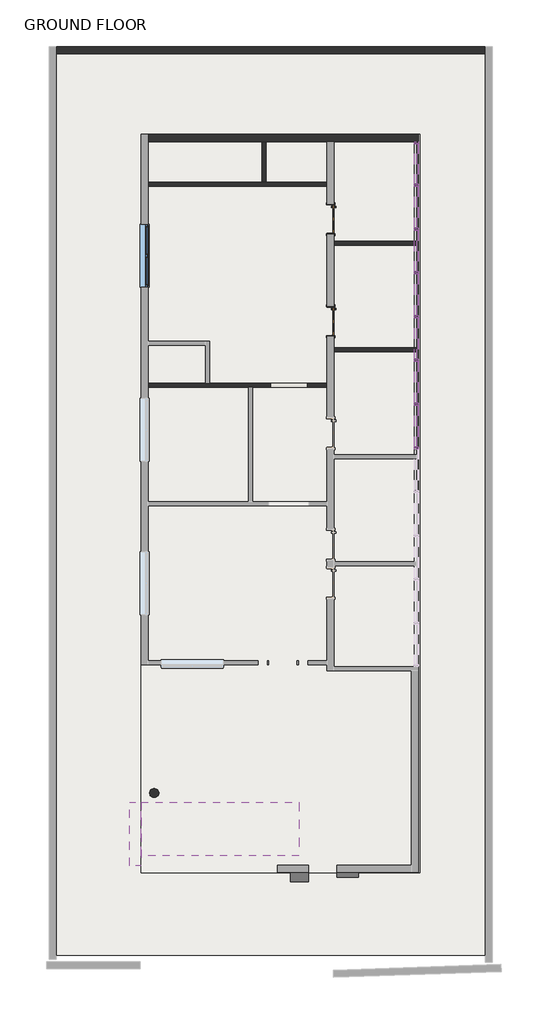
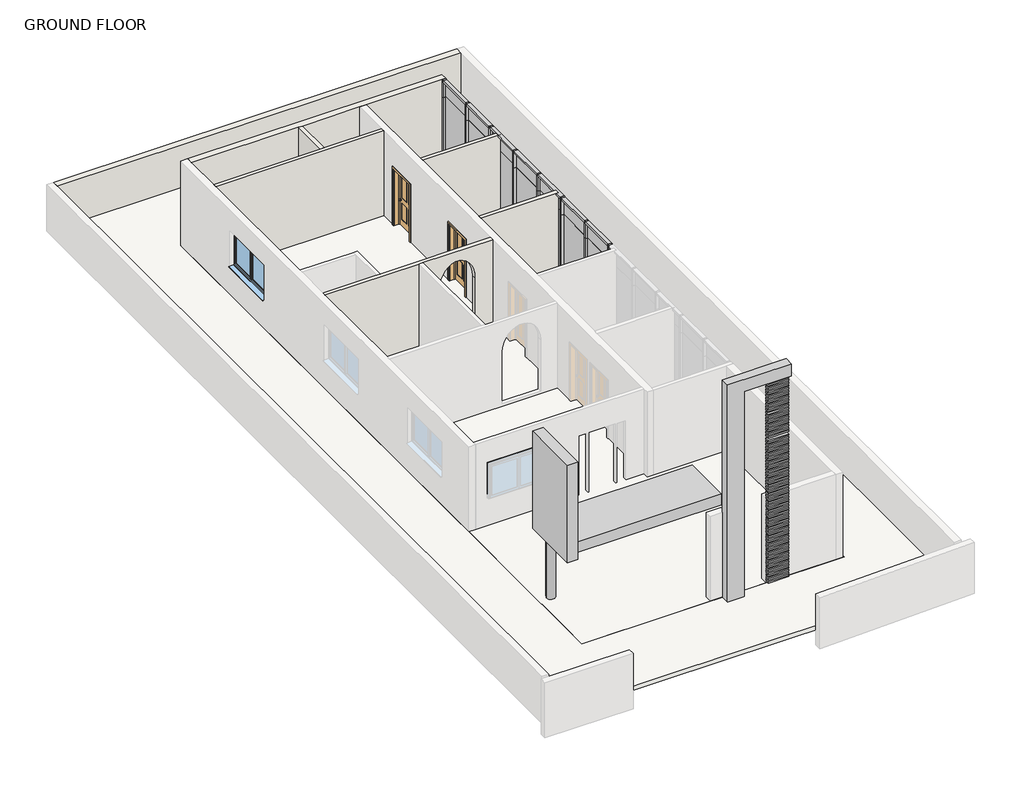
# One storey, part 2 of 2: 31 members, 14 plates, 7 walls, 4 proxies, 2 doors, 2 slabs, 1 column, 1 window.
"""IFC4 building model written with IfcOpenShell, lengths in millimetres."""

from ifc_helpers import new_model, si_unit, point, frame, origin, origin_with_axes, place, context, project, spatial, polyline, ellipse_curve, trimmed, outline, extrude, faceted_brep, transform, mapped, element, save
from ifc_brep_helpers import plane_surface, extruded_surface, advanced_brep
from components import generic_models_11_generic_models_11_3010cca1, generic_models_13_generic_models_13_f044a1e7, generic_models_2_generic_models_2_70f3bfce, generic_models_3_generic_models_3_1afd715e, round_column_column_1_x_1_3d9dadd9, door_8a5afc22, member_fe35c162, member_c919ac1a, member_f0fea5a5, member_6e77e263, member_47bfaf8a, member_ee409385, system_panel_glazed_23a28a9f, system_panel_glazed_17e06366, system_panel_glazed_701ad94b, system_panel_glazed_1ceb456a, w2_0001_w2_7b90d420

model = new_model("IFC4")

# Units and contexts
model_context = context("Model", 3, world=origin())
ifc_project = project(units=[si_unit("LENGTHUNIT", "METRE", prefix="MILLI")], contexts=[model_context])

# Site, building, storey
site = spatial("IfcSite", under=ifc_project)
building = spatial("IfcBuilding", under=site)
storey = spatial("IfcBuildingStorey", under=building, Name="GROUND FLOOR", Elevation=304.8)

# Proxies
placement = place(None, origin())
generic_models_11_generic_models_11_shape = generic_models_11_generic_models_11_3010cca1(model_context)
element("IfcBuildingElementProxy", 1, Name="Generic Models 11 : Generic Models 11", ObjectType="Generic Models 11 : Generic Models 11", at=placement, inside=storey, context=model_context, shape_type="MappedRepresentation", body=[
    mapped(generic_models_11_generic_models_11_shape, transform((0.0, 0.0, 0.0), x_axis=(1.0, 0.0, 0.0), y_axis=(0.0, 1.0, 0.0), z_axis=(0.0, 0.0, 1.0))),
])
generic_models_13_generic_models_13_shape = generic_models_13_generic_models_13_f044a1e7(model_context)
element("IfcBuildingElementProxy", 2, Name="Generic Models 13 : Generic Models 13", ObjectType="Generic Models 13 : Generic Models 13", at=placement, inside=storey, context=model_context, shape_type="MappedRepresentation", body=[
    mapped(generic_models_13_generic_models_13_shape, transform((0.0, 0.0, 0.0), x_axis=(1.0, 0.0, 0.0), y_axis=(0.0, 1.0, 0.0), z_axis=(0.0, 0.0, 1.0))),
])
generic_models_2_generic_models_2_shape = generic_models_2_generic_models_2_70f3bfce(model_context)
element("IfcBuildingElementProxy", 3, Name="Generic Models 2 : Generic Models 2", ObjectType="Generic Models 2 : Generic Models 2", at=placement, inside=storey, context=model_context, shape_type="MappedRepresentation", body=[
    mapped(generic_models_2_generic_models_2_shape, transform((0.0, 0.0, 0.0), x_axis=(1.0, 0.0, 0.0), y_axis=(0.0, 1.0, 0.0), z_axis=(0.0, 0.0, 1.0))),
])
generic_models_3_generic_models_3_shape = generic_models_3_generic_models_3_1afd715e(model_context)
element("IfcBuildingElementProxy", 4, Name="Generic Models 3 : Generic Models 3", ObjectType="Generic Models 3 : Generic Models 3", at=placement, inside=storey, context=model_context, shape_type="MappedRepresentation", body=[
    mapped(generic_models_3_generic_models_3_shape, transform((0.0, 0.0, 0.0), x_axis=(1.0, 0.0, 0.0), y_axis=(0.0, 1.0, 0.0), z_axis=(0.0, 0.0, 1.0))),
])

# Column
round_column_column_1_x_1_shape = round_column_column_1_x_1_3d9dadd9(model_context)
element("IfcColumn", 5, ObjectType="Round Column : COLUMN 1' X 1'", at=placement, inside=storey, context=model_context, shape_type="MappedRepresentation", body=[
    mapped(round_column_column_1_x_1_shape, transform((1692.4423568, -10961.9073314, 0.0), x_axis=(1.0, 0.0, 0.0), y_axis=(0.0, 1.0, 0.0), z_axis=(0.0, 0.0, 1.0))),
])

# Doors
door_shape = door_8a5afc22(model_context)
element("IfcDoor", 6, ObjectType="Door-Interior-Single-4_Panel-Wood : 36\" x 80\"", at=placement, inside=storey, context=model_context, shape_type="MappedRepresentation", body=[
    mapped(door_shape, transform((7334.4173568, 4100.2926686, 304.8), x_axis=(0.0, -1.0, 0.0), y_axis=(1.0, 0.0, 0.0), z_axis=(0.0, 0.0, 1.0))),
])
element("IfcDoor", 7, ObjectType="Door-Interior-Single-4_Panel-Wood : 36\" x 80\"", at=placement, inside=storey, context=model_context, shape_type="MappedRepresentation", body=[
    mapped(door_shape, transform((7334.4173568, 7364.1926686, 304.8), x_axis=(0.0, -1.0, 0.0), y_axis=(1.0, 0.0, 0.0), z_axis=(0.0, 0.0, 1.0))),
])

# Members
member_shape = member_fe35c162(model_context)
element("IfcMember", 8, ObjectType="Rectangular Mullion : 2.5\" x 5\" rectangular", at=placement, inside=storey, context=model_context, shape_type="MappedRepresentation", body=[
    mapped(member_shape, transform((10074.4423568, 9777.1926686, 304.8), x_axis=(0.0, 0.0, -1.0), y_axis=(-1.0, 0.0, 0.0), z_axis=(0.0, 1.0, 0.0))),
])
element("IfcMember", 9, ObjectType="Rectangular Mullion : 2.5\" x 5\" rectangular", at=placement, inside=storey, context=model_context, shape_type="MappedRepresentation", body=[
    mapped(member_shape, transform((10074.4423568, 8474.384335, 3352.8), x_axis=(0.0, 0.0, 1.0), y_axis=(-1.0, 0.0, 0.0), z_axis=(0.0, -1.0, 0.0))),
])
member_2_shape = member_c919ac1a(model_context)
element("IfcMember", 10, ObjectType="Rectangular Mullion : 2.5\" x 5\" rectangular", at=placement, inside=storey, context=model_context, shape_type="MappedRepresentation", body=[
    mapped(member_2_shape, transform((10074.4423568, 7076.3260017, 3352.8), x_axis=(0.0, 0.0, 1.0), y_axis=(-1.0, 0.0, 0.0), z_axis=(0.0, -1.0, 0.0))),
])
element("IfcMember", 11, ObjectType="Rectangular Mullion : 2.5\" x 5\" rectangular", at=placement, inside=storey, context=model_context, shape_type="MappedRepresentation", body=[
    mapped(member_2_shape, transform((10074.4423568, 5678.2676685, 3352.8), x_axis=(0.0, 0.0, 1.0), y_axis=(-1.0, 0.0, 0.0), z_axis=(0.0, -1.0, 0.0))),
])
element("IfcMember", 12, ObjectType="Rectangular Mullion : 2.5\" x 5\" rectangular", at=placement, inside=storey, context=model_context, shape_type="MappedRepresentation", body=[
    mapped(member_2_shape, transform((10074.4423568, 4280.2093352, 3352.8), x_axis=(0.0, 0.0, 1.0), y_axis=(-1.0, 0.0, 0.0), z_axis=(0.0, -1.0, 0.0))),
])
element("IfcMember", 13, ObjectType="Rectangular Mullion : 2.5\" x 5\" rectangular", at=placement, inside=storey, context=model_context, shape_type="MappedRepresentation", body=[
    mapped(member_2_shape, transform((10074.4423568, 2882.1510019, 3352.8), x_axis=(0.0, 0.0, 1.0), y_axis=(-1.0, 0.0, 0.0), z_axis=(0.0, -1.0, 0.0))),
])
element("IfcMember", 14, ObjectType="Rectangular Mullion : 2.5\" x 5\" rectangular", at=placement, inside=storey, context=model_context, shape_type="MappedRepresentation", body=[
    mapped(member_2_shape, transform((10074.4423568, 1484.0926686, 3352.8), x_axis=(0.0, 0.0, 1.0), y_axis=(-1.0, 0.0, 0.0), z_axis=(0.0, -1.0, 0.0))),
])
element("IfcMember", 15, ObjectType="Rectangular Mullion : 2.5\" x 5\" rectangular", at=placement, inside=storey, context=model_context, shape_type="MappedRepresentation", body=[
    mapped(member_2_shape, transform((10074.4423568, 86.0343353, 3352.8), x_axis=(0.0, 0.0, 1.0), y_axis=(-1.0, 0.0, 0.0), z_axis=(0.0, -1.0, 0.0))),
])
element("IfcMember", 16, ObjectType="Rectangular Mullion : 2.5\" x 5\" rectangular", at=placement, inside=storey, context=model_context, shape_type="MappedRepresentation", body=[
    mapped(member_2_shape, transform((10074.4423568, 8410.884335, 304.8), x_axis=(0.0, 0.0, -1.0), y_axis=(-1.0, 0.0, 0.0), z_axis=(0.0, 1.0, 0.0))),
])
element("IfcMember", 17, ObjectType="Rectangular Mullion : 2.5\" x 5\" rectangular", at=placement, inside=storey, context=model_context, shape_type="MappedRepresentation", body=[
    mapped(member_2_shape, transform((10074.4423568, 7012.8260017, 304.8), x_axis=(0.0, 0.0, -1.0), y_axis=(-1.0, 0.0, 0.0), z_axis=(0.0, 1.0, 0.0))),
])
element("IfcMember", 18, ObjectType="Rectangular Mullion : 2.5\" x 5\" rectangular", at=placement, inside=storey, context=model_context, shape_type="MappedRepresentation", body=[
    mapped(member_2_shape, transform((10074.4423568, 5614.7676685, 304.8), x_axis=(0.0, 0.0, -1.0), y_axis=(-1.0, 0.0, 0.0), z_axis=(0.0, 1.0, 0.0))),
])
element("IfcMember", 19, ObjectType="Rectangular Mullion : 2.5\" x 5\" rectangular", at=placement, inside=storey, context=model_context, shape_type="MappedRepresentation", body=[
    mapped(member_2_shape, transform((10074.4423568, 4216.7093352, 304.8), x_axis=(0.0, 0.0, -1.0), y_axis=(-1.0, 0.0, 0.0), z_axis=(0.0, 1.0, 0.0))),
])
element("IfcMember", 20, ObjectType="Rectangular Mullion : 2.5\" x 5\" rectangular", at=placement, inside=storey, context=model_context, shape_type="MappedRepresentation", body=[
    mapped(member_2_shape, transform((10074.4423568, 2818.6510019, 304.8), x_axis=(0.0, 0.0, -1.0), y_axis=(-1.0, 0.0, 0.0), z_axis=(0.0, 1.0, 0.0))),
])
element("IfcMember", 21, ObjectType="Rectangular Mullion : 2.5\" x 5\" rectangular", at=placement, inside=storey, context=model_context, shape_type="MappedRepresentation", body=[
    mapped(member_2_shape, transform((10074.4423568, 1420.5926686, 304.8), x_axis=(0.0, 0.0, -1.0), y_axis=(-1.0, 0.0, 0.0), z_axis=(0.0, 1.0, 0.0))),
])
element("IfcMember", 22, ObjectType="Rectangular Mullion : 2.5\" x 5\" rectangular", at=placement, inside=storey, context=model_context, shape_type="MappedRepresentation", body=[
    mapped(member_2_shape, transform((10074.4423568, 22.5343353, 304.8), x_axis=(0.0, 0.0, -1.0), y_axis=(-1.0, 0.0, 0.0), z_axis=(0.0, 1.0, 0.0))),
])
member_3_shape = member_f0fea5a5(model_context)
element("IfcMember", 23, ObjectType="Rectangular Mullion : 2.5\" x 5\" rectangular", at=placement, inside=storey, context=model_context, shape_type="MappedRepresentation", body=[
    mapped(member_3_shape, transform((10074.4423568, 8442.634335, 304.8), x_axis=(0.0, -1.0, 0.0), y_axis=(-1.0, 0.0, 0.0), z_axis=(0.0, 0.0, -1.0))),
])
element("IfcMember", 24, ObjectType="Rectangular Mullion : 2.5\" x 5\" rectangular", at=placement, inside=storey, context=model_context, shape_type="MappedRepresentation", body=[
    mapped(member_3_shape, transform((10074.4423568, 7044.5760017, 304.8), x_axis=(0.0, -1.0, 0.0), y_axis=(-1.0, 0.0, 0.0), z_axis=(0.0, 0.0, -1.0))),
])
element("IfcMember", 25, ObjectType="Rectangular Mullion : 2.5\" x 5\" rectangular", at=placement, inside=storey, context=model_context, shape_type="MappedRepresentation", body=[
    mapped(member_3_shape, transform((10074.4423568, 5646.5176685, 304.8), x_axis=(0.0, -1.0, 0.0), y_axis=(-1.0, 0.0, 0.0), z_axis=(0.0, 0.0, -1.0))),
])
element("IfcMember", 26, ObjectType="Rectangular Mullion : 2.5\" x 5\" rectangular", at=placement, inside=storey, context=model_context, shape_type="MappedRepresentation", body=[
    mapped(member_3_shape, transform((10074.4423568, 4248.4593352, 304.8), x_axis=(0.0, -1.0, 0.0), y_axis=(-1.0, 0.0, 0.0), z_axis=(0.0, 0.0, -1.0))),
])
element("IfcMember", 27, ObjectType="Rectangular Mullion : 2.5\" x 5\" rectangular", at=placement, inside=storey, context=model_context, shape_type="MappedRepresentation", body=[
    mapped(member_3_shape, transform((10074.4423568, 2850.4010019, 304.8), x_axis=(0.0, -1.0, 0.0), y_axis=(-1.0, 0.0, 0.0), z_axis=(0.0, 0.0, -1.0))),
])
element("IfcMember", 28, ObjectType="Rectangular Mullion : 2.5\" x 5\" rectangular", at=placement, inside=storey, context=model_context, shape_type="MappedRepresentation", body=[
    mapped(member_3_shape, transform((10074.4423568, 1452.3426686, 304.8), x_axis=(0.0, -1.0, 0.0), y_axis=(-1.0, 0.0, 0.0), z_axis=(0.0, 0.0, -1.0))),
])
element("IfcMember", 29, ObjectType="Rectangular Mullion : 2.5\" x 5\" rectangular", at=placement, inside=storey, context=model_context, shape_type="MappedRepresentation", body=[
    mapped(member_3_shape, transform((10074.4423568, 54.2843353, 304.8), x_axis=(0.0, -1.0, 0.0), y_axis=(-1.0, 0.0, 0.0), z_axis=(0.0, 0.0, -1.0))),
])
member_4_shape = member_6e77e263(model_context)
element("IfcMember", 30, ObjectType="Rectangular Mullion : 2.5\" x 5\" rectangular", at=placement, inside=storey, context=model_context, shape_type="MappedRepresentation", body=[
    mapped(member_4_shape, transform((10074.4423568, 8442.634335, 2743.2), x_axis=(0.0, -1.0, 0.0), y_axis=(-1.0, 0.0, 0.0), z_axis=(0.0, 0.0, -1.0))),
])
element("IfcMember", 31, ObjectType="Rectangular Mullion : 2.5\" x 5\" rectangular", at=placement, inside=storey, context=model_context, shape_type="MappedRepresentation", body=[
    mapped(member_4_shape, transform((10074.4423568, 7044.5760017, 2743.2), x_axis=(0.0, -1.0, 0.0), y_axis=(-1.0, 0.0, 0.0), z_axis=(0.0, 0.0, -1.0))),
])
element("IfcMember", 32, ObjectType="Rectangular Mullion : 2.5\" x 5\" rectangular", at=placement, inside=storey, context=model_context, shape_type="MappedRepresentation", body=[
    mapped(member_4_shape, transform((10074.4423568, 5646.5176685, 2743.2), x_axis=(0.0, -1.0, 0.0), y_axis=(-1.0, 0.0, 0.0), z_axis=(0.0, 0.0, -1.0))),
])
element("IfcMember", 33, ObjectType="Rectangular Mullion : 2.5\" x 5\" rectangular", at=placement, inside=storey, context=model_context, shape_type="MappedRepresentation", body=[
    mapped(member_4_shape, transform((10074.4423568, 4248.4593352, 2743.2), x_axis=(0.0, -1.0, 0.0), y_axis=(-1.0, 0.0, 0.0), z_axis=(0.0, 0.0, -1.0))),
])
element("IfcMember", 34, ObjectType="Rectangular Mullion : 2.5\" x 5\" rectangular", at=placement, inside=storey, context=model_context, shape_type="MappedRepresentation", body=[
    mapped(member_4_shape, transform((10074.4423568, 2850.4010019, 2743.2), x_axis=(0.0, -1.0, 0.0), y_axis=(-1.0, 0.0, 0.0), z_axis=(0.0, 0.0, -1.0))),
])
element("IfcMember", 35, ObjectType="Rectangular Mullion : 2.5\" x 5\" rectangular", at=placement, inside=storey, context=model_context, shape_type="MappedRepresentation", body=[
    mapped(member_4_shape, transform((10074.4423568, 1452.3426686, 2743.2), x_axis=(0.0, -1.0, 0.0), y_axis=(-1.0, 0.0, 0.0), z_axis=(0.0, 0.0, -1.0))),
])
element("IfcMember", 36, ObjectType="Rectangular Mullion : 2.5\" x 5\" rectangular", at=placement, inside=storey, context=model_context, shape_type="MappedRepresentation", body=[
    mapped(member_4_shape, transform((10074.4423568, 54.2843353, 2743.2), x_axis=(0.0, -1.0, 0.0), y_axis=(-1.0, 0.0, 0.0), z_axis=(0.0, 0.0, -1.0))),
])
member_5_shape = member_47bfaf8a(model_context)
element("IfcMember", 37, ObjectType="Rectangular Mullion : 2.5\" x 5\" rectangular", at=placement, inside=storey, context=model_context, shape_type="MappedRepresentation", body=[
    mapped(member_5_shape, transform((10074.4423568, 9840.6926686, 3352.8), x_axis=(0.0, 1.0, 0.0), y_axis=(-1.0, 0.0, 0.0), z_axis=(0.0, 0.0, 1.0))),
])
member_6_shape = member_ee409385(model_context)
element("IfcMember", 38, ObjectType="Rectangular Mullion : 2.5\" x 5\" rectangular", at=placement, inside=storey, context=model_context, shape_type="MappedRepresentation", body=[
    mapped(member_6_shape, transform((10074.4423568, 9840.6926686, 2743.2), x_axis=(0.0, 1.0, 0.0), y_axis=(-1.0, 0.0, 0.0), z_axis=(0.0, 0.0, 1.0))),
])

# Plates
system_panel_glazed_shape = system_panel_glazed_23a28a9f(model_context)
element("IfcPlate", 39, ObjectType="System Panel : Glazed", at=placement, inside=storey, context=model_context, shape_type="MappedRepresentation", body=[
    mapped(system_panel_glazed_shape, transform((10074.4423568, 9125.7885018, 368.3), x_axis=(0.0, -1.0, 0.0), y_axis=(1.0, 0.0, 0.0), z_axis=(0.0, 0.0, 1.0))),
])
system_panel_glazed_2_shape = system_panel_glazed_17e06366(model_context)
element("IfcPlate", 40, ObjectType="System Panel : Glazed", at=placement, inside=storey, context=model_context, shape_type="MappedRepresentation", body=[
    mapped(system_panel_glazed_2_shape, transform((10074.4423568, 9125.7885018, 2743.2), x_axis=(0.0, -1.0, 0.0), y_axis=(1.0, 0.0, 0.0), z_axis=(0.0, 0.0, 1.0))),
])
system_panel_glazed_3_shape = system_panel_glazed_701ad94b(model_context)
element("IfcPlate", 41, ObjectType="System Panel : Glazed", at=placement, inside=storey, context=model_context, shape_type="MappedRepresentation", body=[
    mapped(system_panel_glazed_3_shape, transform((10074.4423568, 7743.6051684, 368.3), x_axis=(0.0, -1.0, 0.0), y_axis=(1.0, 0.0, 0.0), z_axis=(0.0, 0.0, 1.0))),
])
element("IfcPlate", 42, ObjectType="System Panel : Glazed", at=placement, inside=storey, context=model_context, shape_type="MappedRepresentation", body=[
    mapped(system_panel_glazed_3_shape, transform((10074.4423568, 6345.5468351, 368.3), x_axis=(0.0, -1.0, 0.0), y_axis=(1.0, 0.0, 0.0), z_axis=(0.0, 0.0, 1.0))),
])
element("IfcPlate", 43, ObjectType="System Panel : Glazed", at=placement, inside=storey, context=model_context, shape_type="MappedRepresentation", body=[
    mapped(system_panel_glazed_3_shape, transform((10074.4423568, 4947.4885018, 368.3), x_axis=(0.0, -1.0, 0.0), y_axis=(1.0, 0.0, 0.0), z_axis=(0.0, 0.0, 1.0))),
])
element("IfcPlate", 44, ObjectType="System Panel : Glazed", at=placement, inside=storey, context=model_context, shape_type="MappedRepresentation", body=[
    mapped(system_panel_glazed_3_shape, transform((10074.4423568, 3549.4301685, 368.3), x_axis=(0.0, -1.0, 0.0), y_axis=(1.0, 0.0, 0.0), z_axis=(0.0, 0.0, 1.0))),
])
element("IfcPlate", 45, ObjectType="System Panel : Glazed", at=placement, inside=storey, context=model_context, shape_type="MappedRepresentation", body=[
    mapped(system_panel_glazed_3_shape, transform((10074.4423568, 2151.3718352, 368.3), x_axis=(0.0, -1.0, 0.0), y_axis=(1.0, 0.0, 0.0), z_axis=(0.0, 0.0, 1.0))),
])
element("IfcPlate", 46, ObjectType="System Panel : Glazed", at=placement, inside=storey, context=model_context, shape_type="MappedRepresentation", body=[
    mapped(system_panel_glazed_3_shape, transform((10074.4423568, 753.313502, 368.3), x_axis=(0.0, -1.0, 0.0), y_axis=(1.0, 0.0, 0.0), z_axis=(0.0, 0.0, 1.0))),
])
system_panel_glazed_4_shape = system_panel_glazed_1ceb456a(model_context)
element("IfcPlate", 47, ObjectType="System Panel : Glazed", at=placement, inside=storey, context=model_context, shape_type="MappedRepresentation", body=[
    mapped(system_panel_glazed_4_shape, transform((10074.4423568, 7743.6051684, 2743.2), x_axis=(0.0, -1.0, 0.0), y_axis=(1.0, 0.0, 0.0), z_axis=(0.0, 0.0, 1.0))),
])
element("IfcPlate", 48, ObjectType="System Panel : Glazed", at=placement, inside=storey, context=model_context, shape_type="MappedRepresentation", body=[
    mapped(system_panel_glazed_4_shape, transform((10074.4423568, 6345.5468351, 2743.2), x_axis=(0.0, -1.0, 0.0), y_axis=(1.0, 0.0, 0.0), z_axis=(0.0, 0.0, 1.0))),
])
element("IfcPlate", 49, ObjectType="System Panel : Glazed", at=placement, inside=storey, context=model_context, shape_type="MappedRepresentation", body=[
    mapped(system_panel_glazed_4_shape, transform((10074.4423568, 4947.4885018, 2743.2), x_axis=(0.0, -1.0, 0.0), y_axis=(1.0, 0.0, 0.0), z_axis=(0.0, 0.0, 1.0))),
])
element("IfcPlate", 50, ObjectType="System Panel : Glazed", at=placement, inside=storey, context=model_context, shape_type="MappedRepresentation", body=[
    mapped(system_panel_glazed_4_shape, transform((10074.4423568, 3549.4301685, 2743.2), x_axis=(0.0, -1.0, 0.0), y_axis=(1.0, 0.0, 0.0), z_axis=(0.0, 0.0, 1.0))),
])
element("IfcPlate", 51, ObjectType="System Panel : Glazed", at=placement, inside=storey, context=model_context, shape_type="MappedRepresentation", body=[
    mapped(system_panel_glazed_4_shape, transform((10074.4423568, 2151.3718352, 2743.2), x_axis=(0.0, -1.0, 0.0), y_axis=(1.0, 0.0, 0.0), z_axis=(0.0, 0.0, 1.0))),
])
element("IfcPlate", 52, ObjectType="System Panel : Glazed", at=placement, inside=storey, context=model_context, shape_type="MappedRepresentation", body=[
    mapped(system_panel_glazed_4_shape, transform((10074.4423568, 753.313502, 2743.2), x_axis=(0.0, -1.0, 0.0), y_axis=(1.0, 0.0, 0.0), z_axis=(0.0, 0.0, 1.0))),
])

# Slabs
element("IfcSlab", 53, ObjectType="FLOORING 1'", at=placement, inside=storey, context=model_context, shape_type="SweptSolid", body=[
    extrude(outline(polyline([(10188.7423568, 10069.2926686), (10188.7423568, -13514.6073314), (1273.3423568, -13514.6073314), (1273.3423568, 10069.2926686), (10188.7423568, 10069.2926686)])), origin_with_axes(), (0.0, 0.0, 1.0), 304.8),
])
element("IfcSlab", 54, ObjectType="FLOORING 6\" 2", at=placement, inside=storey, context=model_context, shape_type="SweptSolid", body=[
    extrude(outline(polyline([(12277.4002222, 12649.3739596), (12277.4002222, -16154.2260404), (-1438.5997778, -16154.2260404), (-1438.5997778, 12649.3739596), (12277.4002222, 12649.3739596)]), holes=[polyline([(10137.9423568, 10069.2926686), (1273.3423568, 10069.2926686), (1273.3423568, -13501.9073314), (10137.9423568, -13501.9073314), (10137.9423568, 10069.2926686)])]), frame((0.0, 0.0, 152.4), z_axis=(0.0, 0.0, 1.0), x_axis=(1.0, 0.0, 0.0)), (0.0, 0.0, 1.0), 152.4),
])

# Walls
element("IfcWall", 55, ObjectType="INNER WALL 5\"", at=placement, inside=storey, context=model_context, shape_type="SweptSolid", body=[
    extrude(outline(polyline([(7445.5423568, 6665.6926686), (10074.4423568, 6665.6926686), (10074.4423568, 6538.6926686), (7445.5423568, 6538.6926686), (7445.5423568, 6665.6926686)])), frame((0.0, 0.0, 304.8), z_axis=(0.0, 0.0, 1.0), x_axis=(1.0, 0.0, 0.0)), (0.0, 0.0, 1.0), 3048.0),
])
element("IfcWall", 56, ObjectType="INNER WALL 5\"", at=placement, inside=storey, context=model_context, shape_type="SweptSolid", body=[
    extrude(outline(polyline([(7445.5423568, 3249.3926686), (10074.4423568, 3249.3926686), (10074.4423568, 3122.3926686), (7445.5423568, 3122.3926686), (7445.5423568, 3249.3926686)])), frame((0.0, 0.0, 304.8), z_axis=(0.0, 0.0, 1.0), x_axis=(1.0, 0.0, 0.0)), (0.0, 0.0, 1.0), 3048.0),
])
element("IfcWall", 57, ObjectType="INNER WALL 5\"", at=placement, inside=storey, context=model_context, shape_type="Brep", body=[
    faceted_brep([(7216.9423568, 8545.2926686, 304.8), (5261.1423568, 8545.2926686, 304.8), (5134.1423568, 8545.2926686, 304.8), (1501.9423568, 8545.2926686, 304.8), (1501.9423568, 8545.2926686, 3352.8), (5134.1423568, 8545.2926686, 3352.8), (5261.1423568, 8545.2926686, 3352.8), (7216.9423568, 8545.2926686, 3352.8), (7216.9423568, 8418.2926686, 304.8), (7216.9423568, 8418.2926686, 3352.8), (1501.9423568, 8418.2926686, 3352.8), (1501.9423568, 8418.2926686, 304.8)], [[[0, 1, 2, 3, 4, 5, 6, 7]], [[8, 9, 10, 11]], [[3, 2, 1, 0, 8, 11]], [[7, 6, 5, 4, 10, 9]], [[4, 3, 11, 10]], [[0, 7, 9, 8]]]),
])
element("IfcWall", 58, ObjectType="INNER WALL 5\"", at=placement, inside=storey, context=model_context, shape_type="SweptSolid", body=[
    extrude(outline(polyline([(5134.1423568, 8545.2926686), (5134.1423568, 9840.6926686), (5261.1423568, 9840.6926686), (5261.1423568, 8545.2926686), (5134.1423568, 8545.2926686)])), frame((0.0, 0.0, 304.8), z_axis=(0.0, 0.0, 1.0), x_axis=(1.0, 0.0, 0.0)), (0.0, 0.0, 1.0), 3048.0),
])
element("IfcWall", 59, ObjectType="INNER WALL 5\"", at=placement, inside=storey, context=model_context, shape_type="AdvancedBrep", body=[
    advanced_brep(
    [(1501.9423568, 1992.0926686, 304.8), (4702.3423568, 1992.0926686, 304.8), (4829.3423568, 1992.0926686, 304.8), (7216.9423568, 1992.0926686, 304.8), (7216.9423568, 1992.0926686, 3352.8), (4829.3423568, 1992.0926686, 3352.8), (4702.3423568, 1992.0926686, 3352.8), (1501.9423568, 1992.0926686, 3352.8), (6599.4941617, 1992.0926686, 325.8987533), (5405.6941617, 1992.0926686, 325.8987533), (5405.6941617, 1992.0926686, 2186.4487533), (6599.4941617, 1992.0926686, 2186.4487533), (1501.9423568, 2119.0926686, 304.8), (1501.9423568, 2119.0926686, 3352.8), (3330.7423568, 2119.0926686, 3352.8), (3457.7423568, 2119.0926686, 3352.8), (7216.9423568, 2119.0926686, 3352.8), (7216.9423568, 2119.0926686, 304.8), (3457.7423568, 2119.0926686, 304.8), (3330.7423568, 2119.0926686, 304.8), (6599.4941617, 2119.0926686, 325.8987533), (6599.4941617, 2119.0926686, 2186.4487533), (5405.6941617, 2119.0926686, 2186.4487533), (5405.6941617, 2119.0926686, 325.8987533)],
    [
        (0, 1),
        (1, 2),
        (2, 3),
        (3, 4),
        (4, 5),
        (5, 6),
        (6, 7),
        (7, 0),
        (8, 9),
        (9, 10),
        (10, 11, ellipse_curve(frame((6002.5941617, 1992.0926686, 2186.4487533), z_axis=(0.0, 1.0, 0.0), x_axis=(0.0, 0.0, -1.0)), 812.8, 596.9)),
        (11, 8),
        (12, 13),
        (13, 14),
        (14, 15),
        (15, 16),
        (16, 17),
        (17, 18),
        (18, 19),
        (19, 12),
        (20, 21),
        (21, 22, ellipse_curve(frame((6002.5941617, 2119.0926686, 2186.4487533), z_axis=(0.0, -1.0, 0.0), x_axis=(0.0, 0.0, -1.0)), 812.8, 596.9)),
        (22, 23),
        (23, 20),
        (7, 13),
        (12, 0),
        (3, 17),
        (16, 4),
        (8, 20),
        (23, 9),
        (22, 10),
        (21, 11),
    ],
    [
        plane_surface(frame((1501.9423568, 1992.0926686, 304.8), z_axis=(0.0, -1.0, 0.0), x_axis=(1.0, 0.0, 0.0))),
        plane_surface(frame((1501.9423568, 2119.0926686, 304.8), z_axis=(0.0, 1.0, 0.0), x_axis=(-1.0, 0.0, 0.0))),
        plane_surface(frame((1501.9423568, -8333.0073314, 304.8), z_axis=(-1.0, 0.0, 0.0), x_axis=(0.0, 1.0, 0.0))),
        plane_surface(frame((7216.9423568, 9954.9926686, 304.8), z_axis=(1.0, 0.0, 0.0), x_axis=(0.0, -1.0, 0.0))),
        plane_surface(frame((1387.6423568, 1992.0926686, 304.8), z_axis=(0.0, 0.0, -1.0), x_axis=(0.0, 1.0, 0.0))),
        plane_surface(frame((7331.2423568, 1992.0926686, 3352.8), z_axis=(0.0, 0.0, 1.0), x_axis=(0.0, 1.0, 0.0))),
        plane_surface(frame((6599.4941617, 1992.0926686, 325.8987533), z_axis=(0.0, 0.0, 1.0), x_axis=(0.0, 1.0, 0.0))),
        plane_surface(frame((5405.6941617, 1992.0926686, 325.8987533), z_axis=(1.0, 0.0, 0.0), x_axis=(0.0, 1.0, 0.0))),
        extruded_surface(trimmed(ellipse_curve(frame((6002.5941617, 2182.5926686, 2186.4487533), z_axis=(0.0, 1.0, 0.0), x_axis=(1.0, 0.0, 0.0)), 596.9, 812.8), [point((5405.6941617, 2182.5926686, 2186.4487533))], [point((6599.4941617, 2182.5926686, 2186.4487533))], True, "CARTESIAN"), (0.0, -127.0, 0.0), 127.0),
        plane_surface(frame((6599.4941617, 1992.0926686, 2186.4487533), z_axis=(-1.0, 0.0, 0.0), x_axis=(0.0, 1.0, 0.0))),
    ],
    [
        (0, [[1, 2, 3, 4, 5, 6, 7, 8], [9, 10, 11, 12]]),
        (1, [[13, 14, 15, 16, 17, 18, 19, 20], [21, 22, 23, 24]]),
        (2, [[-8, 25, -13, 26]]),
        (3, [[-4, 27, -17, 28]]),
        (4, [[-3, -2, -1, -26, -20, -19, -18, -27]]),
        (5, [[-7, -6, -5, -28, -16, -15, -14, -25]]),
        (6, [[-9, 29, -24, 30]]),
        (7, [[-10, -30, -23, 31]]),
        (8, [[-11, -31, -22, 32]]),
        (9, [[-12, -32, -21, -29]]),
    ],
),
])
element("IfcWall", 60, ObjectType="OUTER WALL 9\"", at=placement, inside=storey, context=model_context, shape_type="Brep", body=[
    faceted_brep([(1501.9423568, 9840.6926686, 304.8), (5134.1423568, 9840.6926686, 304.8), (5261.1423568, 9840.6926686, 304.8), (7216.9423568, 9840.6926686, 304.8), (7445.5423568, 9840.6926686, 304.8), (10137.9423568, 9840.6926686, 304.8), (10137.9423568, 9840.6926686, 3352.8), (7445.5423568, 9840.6926686, 3352.8), (7216.9423568, 9840.6926686, 3352.8), (5261.1423568, 9840.6926686, 3352.8), (5134.1423568, 9840.6926686, 3352.8), (1501.9423568, 9840.6926686, 3352.8), (1501.9423568, 10069.2926686, 304.8), (1501.9423568, 10069.2926686, 3352.8), (10137.9423568, 10069.2926686, 3352.8), (10137.9423568, 10069.2926686, 304.8)], [[[0, 1, 2, 3, 4, 5, 6, 7, 8, 9, 10, 11]], [[12, 13, 14, 15]], [[5, 4, 3, 2, 1, 0, 12, 15]], [[6, 5, 15, 14]], [[11, 10, 9, 8, 7, 6, 14, 13]], [[0, 11, 13, 12]]]),
])
element("IfcWall", 61, ObjectType="OUTER WALL 9\"", at=placement, inside=storey, context=model_context, shape_type="Brep", body=[
    faceted_brep([(12277.4002222, 12877.9739596, 0.0), (-1438.5997778, 12877.9739596, 0.0), (-1438.5997778, 12877.9739596, 152.4), (-1438.5997778, 12877.9739596, 1828.8), (12277.4002222, 12877.9739596, 1828.8), (12277.4002222, 12649.3739596, 0.0), (12277.4002222, 12649.3739596, 1828.8), (-1438.5997778, 12649.3739596, 1828.8), (-1438.5997778, 12649.3739596, 0.0)], [[[0, 1, 2, 3, 4]], [[5, 6, 7, 8]], [[1, 0, 5, 8]], [[4, 3, 7, 6]], [[3, 2, 1, 8, 7]], [[0, 4, 6, 5]]]),
])

# Window
w2_0001_w2_shape = w2_0001_w2_7b90d420(model_context)
element("IfcWindow", 62, ObjectType="w2.0001 : w2", at=placement, inside=storey, context=model_context, shape_type="MappedRepresentation", body=[
    mapped(w2_0001_w2_shape, transform((1387.6423568, 6195.7926686, 304.8), x_axis=(0.0, 1.0, 0.0), y_axis=(-1.0, 0.0, 0.0), z_axis=(0.0, 0.0, 1.0))),
])

save(model, "model.ifc")

# Revit data of these elements
# Type "Round Column : COLUMN 1' X 1'"
#   Assembly Code = "B1010200"
#   Diameter = 1' - 0"
#   Offset Base = 0' - 0"
#   Offset Top = 0' - 0"
#   Material = CREAM BEIGE COLOUR
# Type "Door-Interior-Single-4_Panel-Wood : 36\" x 80\""
#   Type Mark = "9"
#   Assembly Code = "C1020300"
#   Analytic Construction = "Wooden"
#   Top Rail = 0' - 4 11/16"
#   Thickness = 0' - 1 3/8"
#   Thermal Resistance (R) = 2.5876 (h·ft²·°F)/BTU
#   Swing Angle [instance default] = 90.00°
#   Stiles = 0' - 4 3/4"
#   Rough Width = 3' - 2"
#   Rough Height = 6' - 9"
#   Mullion = 0' - 4 1/2"
#   Lock Rail = 0' - 7 1/2"
#   Height = 6' - 8"
#   Width = 3' - 0"
#   Heat Transfer Coefficient (U) = 0.3865 BTU/(h·ft²·°F)
#   Bottom Rail = 0' - 9 1/8"
#   Trim Material = Cherry
#   Panel Material = Cherry
#   Frame Material = Cherry
#   Door Handle Material = Aluminum
#   Visual Light Transmittance = 0
#   Solar Heat Gain Coefficient = 0
#   Wall Closure = (empty or 0)
#   Function = (empty or 0)
# Type "Rectangular Mullion : 2.5\" x 5\" rectangular"
#   built-in parameter 1007304 = 0.416667 (stored number, unit not read)
#   built-in parameter 1007301 = 0.104167 (stored number, unit not read)
#   built-in parameter 1007300 = 0.104167 (stored number, unit not read)
# Type "System Panel : Glazed"
#   Construction Type Id = "GSP4R"
#   Analytic Construction = "1/8 in Pilkington single glazing"
#   Visual Light Transmittance = 0.9
#   Solar Heat Gain Coefficient = 0.86
#   Heat Transfer Coefficient (U) = 1.18115 BTU/(h·ft²·°F)
#   Define Thermal Properties by = 1
# Type "FLOORING 1'"
#   Assembly Code = "B1010"
#   Function = 0
#   Layers, outside or top first: 1' - 0" "CARPET MATERIAL FLOORING" (function 1)
# Type "FLOORING 6\" 2"
#   Assembly Code = "B1010"
#   Function = 0
#   Layers, outside or top first: 0' - 6" "CARPET MATERIAL FLOORING(1)" (function 1)
# Type "INNER WALL 5\""
#   Assembly Code = "B2010"
#   Layers, outside or top first: 0' - 5" "CREAM BEIGE COLOUR" (function 1)
# Type "OUTER WALL 9\""
#   Assembly Code = "B2010"
#   Layers, outside or top first: 0' - 9" "CREAM BEIGE COLOUR" (function 1)
# Type "w2.0001 : w2"
#   Type Mark = "19"
#   Operation = "DoublePanelVertical"
#   Keynote = "16.05.01"
#   Analytic Construction = "<None>"
#   Rough Width = 6' - 7.13386"
#   Rough Height = 4' - 1.6063"
#   Rahmentiefe = 0' - 2.3622"
#   Rahmenhöhe unten = 0' - 3.14961"
#   Rahmehöhe oben = 0' - 3.14961"
#   Rahmenbreite = 0' - 2.3622"
#   Height = 4' - 1.6063"
#   Flügeltiefe = 0' - 2.3622"
#   Flügelbreite = 0' - 2.3622"
#   Einbautiefe (von außen) [instance default] = 0' - 5.51181"
#   Width = 6' - 7.13386"
#   Kippflügel [instance default] = yes
#   Drehflügel im Grundriß darstellen [instance default] = no
#   Drehflügel [instance default] = yes
#   Define Thermal Properties by = 1
#   Rahmen [instance default] = none
#   Glas [instance default] = none
#   Flügel [instance default] = none
#   Fensterbank aussen [instance default] = none
#   Fensterbank innen [instance default] = none
#   Wall Closure = (empty or 0)
# Element 1 (IfcBuildingElementProxy, "Generic Models 11 : Generic Models 11")
#   Phase Created = New Construction
#   Materials on its faces: "Clad - White"
# Element 2 (IfcBuildingElementProxy, "Generic Models 13 : Generic Models 13")
#   Phase Created = New Construction
#   Materials on its faces: "Clad - White"
# Element 3 (IfcBuildingElementProxy, "Generic Models 2 : Generic Models 2")
#   Phase Created = New Construction
#   Materials on its faces: "Clad - White"
# Element 4 (IfcBuildingElementProxy, "Generic Models 3 : Generic Models 3")
#   Phase Created = New Construction
#   Materials on its faces: "WOOD MATERIAL 9\""
# Element 5 (IfcColumn, "Round Column : COLUMN 1' X 1'")
#   Phase Created = New Construction
#   Materials on its faces: "CREAM BEIGE COLOUR"
# Elements 6, 7 (IfcDoor, "Door-Interior-Single-4_Panel-Wood : 36\" x 80\"")
#   Swing Angle = 90.00°
#   Phase Created = New Construction
#   Materials on its faces: "Cherry", "Aluminum"
# Elements 8, 9, 10, 11, 12, 13, 14, 15, 16, 17, 18, 19, 20, 21, 22, 23, 24, 25, 26, 27, 28, 29, 30, 31, 32, 33, 34, 35, 36, 37, 38 (IfcMember, "Rectangular Mullion : 2.5\" x 5\" rectangular")
#   Phase Created = New Construction
#   Materials on its faces: "BLACK MATERIAL"
# Elements 39, 40, 41, 42, 43, 44, 45, 46, 47, 48, 49, 50, 51, 52 (IfcPlate, "System Panel : Glazed")
#   Phase Created = New Construction
#   Materials on its faces: "Glass"
# Element 53 (IfcSlab, "FLOORING 1'")
#   Height Offset From Level = 0' - 0"
#   Phase Created = New Construction
#   Materials on its faces: "CARPET MATERIAL FLOORING"
# Element 54 (IfcSlab, "FLOORING 6\" 2")
#   Height Offset From Level = 0' - 0"
#   Phase Created = New Construction
#   Materials on its faces: "CARPET MATERIAL FLOORING(1)"
# Element 55 (IfcWall, "INNER WALL 5\"")
#   Top Offset = 0' - 0"
#   Base Offset = 0' - 0"
#   Unconnected Height = 10' - 0"
#   wall height = 10' - 0"
#   Phase Created = New Construction
#   Base Constraint = GROUND FLOOR
#   Materials on its faces: "CREAM BEIGE COLOUR"
# Elements 56, 57, 58, 59 (IfcWall, "INNER WALL 5\"")
#   Top Offset = 0' - 0"
#   Base Offset = 0' - 0"
#   wall height = 10' - 0"
#   Phase Created = New Construction
#   Base Constraint = GROUND FLOOR
#   Top Constraint = FIRST FLOOR
#   Materials on its faces: "CREAM BEIGE COLOUR"
# Element 60 (IfcWall, "OUTER WALL 9\"")
#   Top Offset = 0' - 0"
#   Base Offset = 0' - 0"
#   Unconnected Height = 10' - 0"
#   wall height = 10' - 0"
#   Phase Created = New Construction
#   Base Constraint = GROUND FLOOR
#   Materials on its faces: "CREAM BEIGE COLOUR"
# Element 61 (IfcWall, "OUTER WALL 9\"")
#   built-in parameter 1001111 = -1' - 0"
#   Top Offset = 0' - 0"
#   Base Offset = -1' - 0"
#   Unconnected Height = 6' - 0"
#   wall height = 6' - 0"
#   Phase Created = New Construction
#   Base Constraint = GROUND FLOOR
#   Materials on its faces: "CREAM BEIGE COLOUR"
# Element 62 (IfcWindow, "w2.0001 : w2")
#   Mark = "4"
#   Einbautiefe (von außen) = 0' - 5.51181"
#   Kippflügel = yes
#   Drehflügel im Grundriß darstellen = no
#   Drehflügel = yes
#   Rahmen = none
#   Glas = none
#   Flügel = none
#   Fensterbank innen = none
#   Fensterbank aussen = none
#   Phase Created = New Construction
#   Materials on its faces: "Fenster - Kunststoff", "Fenster - Kunststoff weiss", "Glass", "Fenster - Holz"
# Materials
#   "CREAM BEIGE COLOUR": class "Generic", colour RGB 120 120 120, transparency 0, Cost = 0
#   "Cherry": class "Wood", colour RGB 226 177 128, transparency 0, Description = "Prunus Serotina", Cost = 0
#   "Aluminum": class "Metal", colour RGB 247 247 247, transparency 0, Description = "Aluminum 6061", Cost = 0
#   "CARPET MATERIAL FLOORING": class "Generic", colour RGB 120 120 120, transparency 0, Cost = 0
#   "CARPET MATERIAL FLOORING(1)": class "Generic", colour RGB 120 120 120, transparency 0, Cost = 0
#   "Clad - White": class "Wood", colour RGB 242 242 238, transparency 0, Cost = 0
#   "WOOD MATERIAL 9\"": class "Generic", colour RGB 120 120 120, transparency 0, Cost = 0
#   "BLACK MATERIAL": class "Generic", colour RGB 120 120 120, transparency 0, Cost = 0
#   "Glass": class "Glass", colour RGB 0 128 192, transparency 0.75, Description = "Soda Lime Glass", Cost = 0
#   "Fenster - Kunststoff": colour RGB 249 249 249, transparency 0
#   "Fenster - Kunststoff weiss": colour RGB 249 249 249, transparency 0
#   "Fenster - Holz": colour RGB 216 135 75, transparency 0
